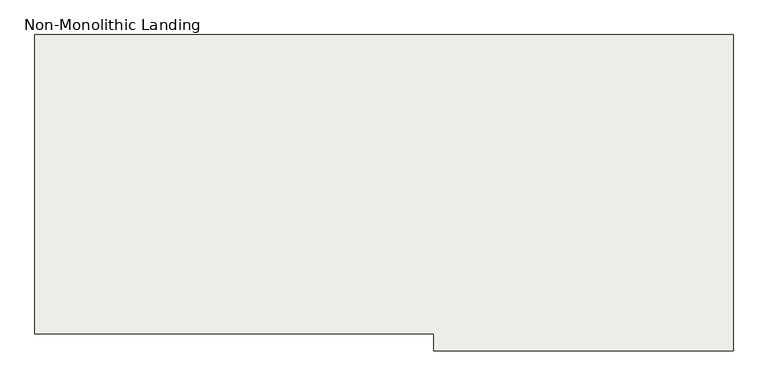
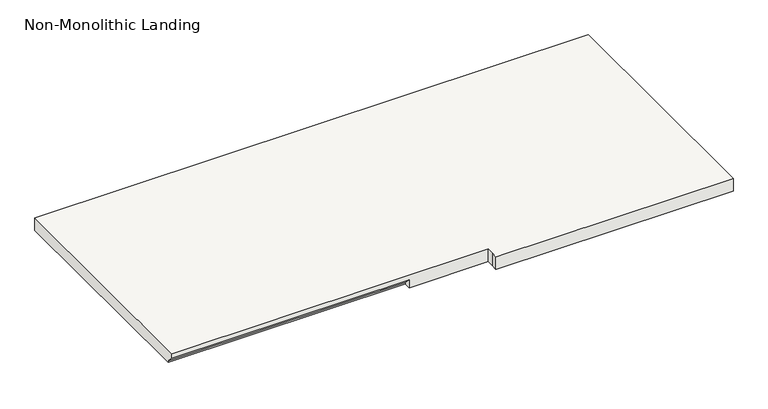
"""IFC4 building model written with IfcOpenShell, lengths in millimetres: slab geometry, Non-Monolithic Landing."""

from ifc_helpers import new_model, si_unit, origin, place, context, project, spatial, faceted_brep, source, transform, mapped, element, save


def non_monolithic_landing_7206712e(model_context):
    return source(origin(), model_context, "Body", "Brep", [
        faceted_brep([(7464.4260838, 825.5660813, 8769.35), (7464.4260838, 850.9660813, 8743.95), (8378.8260838, 850.9660813, 8743.95), (8378.8260838, 825.5660813, 8769.35), (8683.6260838, 825.5660813, 8788.4), (8683.6260838, 798.8027016, 8788.4), (8683.6260838, 773.4027016, 8788.4), (9598.0260838, 773.4027016, 8788.4), (9598.0260838, 798.8027016, 8788.4), (9598.0260838, 1739.9660813, 8788.4), (7464.4260838, 1739.9660813, 8788.4), (7464.4260838, 825.5660813, 8788.4), (8378.8260838, 850.9660813, 8737.6), (7464.4260838, 850.9660813, 8737.6), (7464.4260838, 1739.9660813, 8737.6), (9598.0260838, 1739.9660813, 8737.6), (9598.0260838, 798.8027016, 8737.6), (9598.0260838, 773.4027016, 8737.6), (8683.6260838, 773.4027016, 8737.6), (8683.6260838, 798.8027016, 8737.6), (8683.6260838, 825.5660813, 8737.6), (8378.8260838, 825.5660813, 8737.6)], [[[0, 1, 2, 3]], [[4, 5, 6, 7, 8, 9, 10, 11]], [[12, 13, 14, 15, 16, 17, 18, 19, 20, 21]], [[13, 12, 2, 1]], [[12, 21, 3, 2]], [[4, 11, 0, 3, 21, 20]], [[5, 4, 20, 19]], [[6, 5, 19, 18]], [[7, 6, 18, 17]], [[8, 7, 17, 16]], [[9, 8, 16, 15]], [[10, 9, 15, 14]], [[11, 10, 14, 13, 1, 0]]]),
    ])


if __name__ == "__main__":
    model = new_model("IFC4")
    model_context = context("Model", 3, world=origin())
    ifc_project = project(units=[si_unit("LENGTHUNIT", "METRE", prefix="MILLI")], contexts=[model_context])
    site = spatial("IfcSite", under=ifc_project)
    building = spatial("IfcBuilding", under=site)
    placement = place(None, origin())
    non_monolithic_landing_shape = non_monolithic_landing_7206712e(model_context)
    element("IfcSlab", 1, ObjectType="Non-Monolithic Landing", at=placement, inside=building, context=model_context, shape_type="MappedRepresentation", body=[
        mapped(non_monolithic_landing_shape, transform((0.0, 0.0, 0.0), x_axis=(1.0, 0.0, 0.0), y_axis=(0.0, 1.0, 0.0), z_axis=(0.0, 0.0, 1.0))),
    ])
    save(model, "model.ifc")
